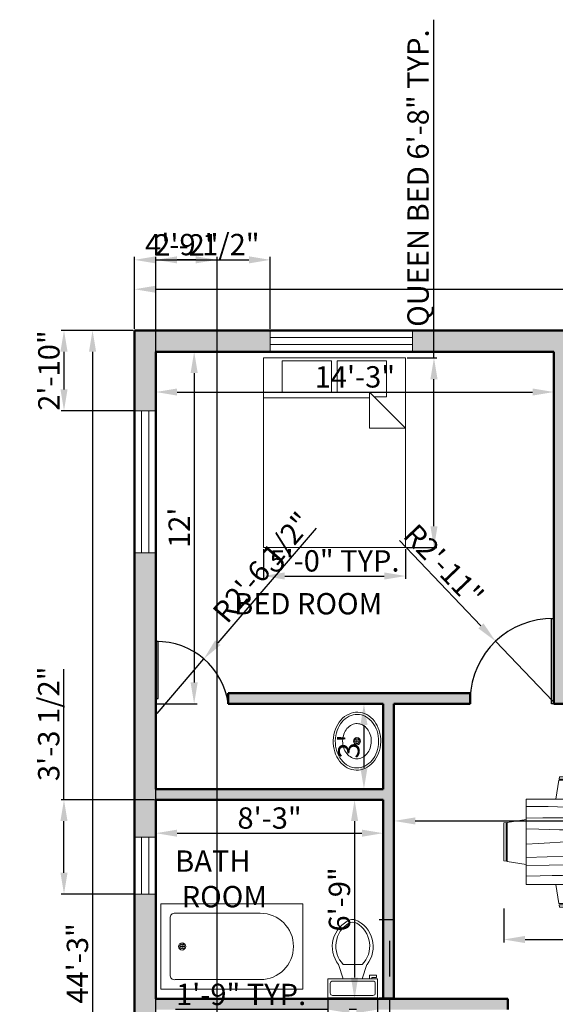
# Model space of a CAD drawing. Units: inches. Extents: x 875413 to 876020, y 447446 to 448210.
# Tile 5 of 8: x 875413 to 875639, y 447795 to 448210. Entities that reach past the tile are written whole.
import ezdxf

# ---------------------------------------------------------------- set-up
doc = ezdxf.new("R2010")
doc.units = ezdxf.units.IN
for name, color, linetype, lineweight in [('A-ANNO-DIMS', 2, 'Continuous', 13), ('A-AREA-IDEN', 7, 'Continuous', 25), ('A-DOOR', 3, 'Continuous', 25), ('A-FLOR-FIXT', 9, 'Continuous', 18), ('A-FURN', 8, 'Continuous', 18), ('A-GLAZ', 4, 'Continuous', 20), ('A-WALL', 7, 'Continuous', 50)]:
    doc.layers.add(name, color=color, linetype=linetype, lineweight=lineweight)
doc.layers.add('A-WALL-PATT', color=18, linetype='Continuous', lineweight=13, true_color=0x000000)
doc.styles.get("Standard").update_dxf_attribs({"font": 'arial.ttf'})
doc.dimstyles.new('ISO-25', dxfattribs={"dimtxt": 9, "dimasz": 9, "dimexe": 1.25, "dimexo": 0.625, "dimtad": 1, "dimdec": 1, "dimrnd": 9, "dimlunit": 3, "dimtxsty": 'Standard', "dimcen": 2.5, "dimadec": 0, "dimazin": 0, "dimtfac": 1, "dimtdec": 1, "dimtmove": 0, "dimatfit": 3, "dimfxl": 1, "dimarcsym": 0})

# ---------------------------------------------------------------- blocks, each defined once
blk = doc.blocks.new('*D1')
at = {"layer": 'A-ANNO-DIMS', "color": 0, "lineweight": -2, "transparency": 16777216}
for p, q in [((875470.7, 448069.39), (875470.7, 448051.77)), ((875638.7, 448069.39), (875638.7, 448051.77)), ((875479.7, 448053.02), (875629.7, 448053.02))]:
    blk.add_line(p, q, dxfattribs=at)
at = {"layer": 'A-ANNO-DIMS', "color": 0, "transparency": 16777216}
for points in [[(875479.7, 448054.52), (875479.7, 448051.52), (875470.7, 448053.02)], [(875629.7, 448054.52), (875629.7, 448051.52), (875638.7, 448053.02)]]:
    blk.add_solid(points, dxfattribs=at)
at = {"layer": 'Defpoints', "color": 0, "transparency": 16777216}
for p in [(875470.7, 448070.02), (875638.7, 448070.02), (875638.7, 448053.02)]:
    blk.add_point(p, dxfattribs=at)
at = {"layer": 'A-ANNO-DIMS', "color": 0, "transparency": 16777216, "insert": (875554.7, 448058.25), "char_height": 9, "attachment_point": 5}
blk.add_mtext('14\'-3"', dxfattribs=at)
blk = doc.blocks.new('*D2')
at = {"layer": 'A-ANNO-DIMS', "color": 0, "lineweight": -2, "transparency": 16777216}
for p, q in [((875471.33, 448070.02), (875488.13, 448070.02)), ((875486.88, 448061.02), (875486.88, 447930.52)), ((875471.33, 447921.52), (875488.13, 447921.52))]:
    blk.add_line(p, q, dxfattribs=at)
at = {"layer": 'A-ANNO-DIMS', "color": 0, "transparency": 16777216}
for points in [[(875485.38, 448061.02), (875488.38, 448061.02), (875486.88, 448070.02)], [(875485.38, 447930.52), (875488.38, 447930.52), (875486.88, 447921.52)]]:
    blk.add_solid(points, dxfattribs=at)
at = {"layer": 'Defpoints', "color": 0, "transparency": 16777216}
for p in [(875470.7, 448070.02), (875470.7, 447921.52), (875486.88, 447921.52)]:
    blk.add_point(p, dxfattribs=at)
at = {"layer": 'A-ANNO-DIMS', "color": 0, "transparency": 16777216, "insert": (875481.73, 447995.77), "char_height": 9, "attachment_point": 5, "rotation": 90}
blk.add_mtext("12'", dxfattribs=at)
blk = doc.blocks.new('*D7')
at = {"layer": 'A-ANNO-DIMS', "color": 0, "lineweight": -2, "transparency": 16777216}
for p, q in [((875566.08, 447921.52), (875557.28, 447921.52)), ((875558.53, 447912.52), (875558.53, 447894.52)), ((875566.08, 447885.52), (875557.28, 447885.52))]:
    blk.add_line(p, q, dxfattribs=at)
at = {"layer": 'A-ANNO-DIMS', "color": 0, "transparency": 16777216}
for points in [[(875557.03, 447912.52), (875560.03, 447912.52), (875558.53, 447921.52)], [(875557.03, 447894.52), (875560.03, 447894.52), (875558.53, 447885.52)]]:
    blk.add_solid(points, dxfattribs=at)
at = {"layer": 'Defpoints', "color": 0, "transparency": 16777216}
for p in [(875566.7, 447921.52), (875558.53, 447885.52), (875566.7, 447885.52)]:
    blk.add_point(p, dxfattribs=at)
at = {"layer": 'A-ANNO-DIMS', "color": 0, "transparency": 16777216, "insert": (875553.31, 447903.52), "char_height": 9, "attachment_point": 5, "rotation": 90}
blk.add_mtext("3'", dxfattribs=at)
blk = doc.blocks.new('*D8')
at = {"layer": 'A-ANNO-DIMS', "color": 0, "lineweight": -2, "transparency": 16777216}
for p, q in [((875566.08, 447881.02), (875553.32, 447881.02)), ((875554.57, 447872.02), (875554.57, 447806.02)), ((875566.08, 447797.02), (875553.32, 447797.02))]:
    blk.add_line(p, q, dxfattribs=at)
at = {"layer": 'A-ANNO-DIMS', "color": 0, "transparency": 16777216}
for points in [[(875553.07, 447872.02), (875556.07, 447872.02), (875554.57, 447881.02)], [(875553.07, 447806.02), (875556.07, 447806.02), (875554.57, 447797.02)]]:
    blk.add_solid(points, dxfattribs=at)
at = {"layer": 'Defpoints', "color": 0, "transparency": 16777216}
for p in [(875566.7, 447881.02), (875554.57, 447797.02), (875566.7, 447797.02)]:
    blk.add_point(p, dxfattribs=at)
at = {"layer": 'A-ANNO-DIMS', "color": 0, "transparency": 16777216, "insert": (875549.35, 447839.02), "char_height": 9, "attachment_point": 5, "rotation": 90}
blk.add_mtext('6\'-9"', dxfattribs=at)
blk = doc.blocks.new('*D9')
at = {"layer": 'A-ANNO-DIMS', "color": 0, "lineweight": -2, "transparency": 16777216}
for p, q in [((875470.7, 447880.39), (875470.7, 447865.69)), ((875566.7, 447880.39), (875566.7, 447865.69)), ((875479.7, 447866.94), (875557.7, 447866.94))]:
    blk.add_line(p, q, dxfattribs=at)
at = {"layer": 'A-ANNO-DIMS', "color": 0, "transparency": 16777216}
for points in [[(875479.7, 447868.44), (875479.7, 447865.44), (875470.7, 447866.94)], [(875557.7, 447868.44), (875557.7, 447865.44), (875566.7, 447866.94)]]:
    blk.add_solid(points, dxfattribs=at)
at = {"layer": 'Defpoints', "color": 0, "transparency": 16777216}
for p in [(875470.7, 447881.02), (875566.7, 447881.02), (875566.7, 447866.94)]:
    blk.add_point(p, dxfattribs=at)
at = {"layer": 'A-ANNO-DIMS', "color": 0, "transparency": 16777216, "insert": (875518.7, 447872.16), "char_height": 9, "attachment_point": 5}
blk.add_mtext('8\'-3"', dxfattribs=at)
blk = doc.blocks.new('*D13')
at = {"layer": 'A-ANNO-DIMS', "color": 0, "lineweight": -2, "transparency": 16777216}
for p, q in [((875571.2, 447920.89), (875571.2, 447870.86)), ((875838.2, 447920.89), (875838.2, 447870.86)), ((875580.2, 447872.11), (875829.2, 447872.11))]:
    blk.add_line(p, q, dxfattribs=at)
at = {"layer": 'A-ANNO-DIMS', "color": 0, "transparency": 16777216}
for points in [[(875580.2, 447873.61), (875580.2, 447870.61), (875571.2, 447872.11)], [(875829.2, 447873.61), (875829.2, 447870.61), (875838.2, 447872.11)]]:
    blk.add_solid(points, dxfattribs=at)
at = {"layer": 'Defpoints', "color": 0, "transparency": 16777216}
for p in [(875571.2, 447921.52), (875838.2, 447921.52), (875838.2, 447872.11)]:
    blk.add_point(p, dxfattribs=at)
at = {"layer": 'A-ANNO-DIMS', "color": 0, "transparency": 16777216, "insert": (875704.7, 447877.33), "char_height": 9, "attachment_point": 5}
blk.add_mtext('22\'-6"', dxfattribs=at)
blk = doc.blocks.new('Bed - Queen')
for p, q in [((0, -80.00003), (0, 0)), ((0, 0), (59.99999, 0)), ((59.99999, 0), (59.99999, -80.00003)), ((7.99999, -1.2), (28.79998, -1.2)), ((7.99999, -14.4), (7.99999, -1.2)), ((28.79998, -1.2), (28.79998, -14.4)), ((31.19999, -1.2), (51.99999, -1.2)), ((31.19999, -14.4), (31.19999, -1.2)), ((51.99999, -1.2), (51.99999, -16.4)), ((0, -14.4), (44.8, -14.4)), ((59.99999, -29.6), (44.8, -14.4)), ((44.8, -14.4), (44.8, -29.6)), ((51.99999, -16.4), (46.79936, -16.4)), ((44.8, -16.8), (0, -16.8)), ((44.8, -29.6), (59.99999, -29.6)), ((59.99999, -80.00003), (0, -80.00003))]:
    blk.add_line(p, q)
blk = doc.blocks.new('Dining Set - 36 x 72 in.')
for p, q in [((-22.2343, 26.00059), (-23.4847, 17.99762)), ((-22.2304, 26), (-5.7608, 26)), ((-22, 27.5), (-22.1562, 26.50042)), ((-5.8416, 26.5), (-22.1534, 26.5)), ((-22, 27.5), (-6, 27.5)), ((-5.8437, 26.49966), (-6, 27.5)), ((-4.5152, 17.99762), (-5.7655, 25.99926)), ((5.7657, 26.00059), (4.5153, 17.99762)), ((5.7696, 26), (22.2392, 26)), ((6, 27.5), (5.8438, 26.50042)), ((22.1584, 26.5), (5.8466, 26.5)), ((6, 27.5), (22, 27.5)), ((22.1563, 26.49966), (22, 27.5)), ((23.4848, 17.99762), (22.2345, 25.99926)), ((36, 18), (-36, 18)), ((-36, 18), (-36, -18)), ((36, -18), (36, 18)), ((-44.0006, 8.23428), (-35.9976, 9.48474)), ((44.0006, 8.23428), (35.9976, 9.48474)), ((-45.5, 8), (-44.5004, 8.15617)), ((-45.5, 8), (-45.5, -8)), ((-44.5, -8.15843), (-44.5, 8.15338)), ((-44, 8.23041), (-44, -8.23915)), ((44, 8.23041), (44, -8.23915)), ((44.5, -8.15843), (44.5, 8.15338)), ((45.5, 8), (44.5005, 8.15617)), ((45.5, 8), (45.5, -8)), ((-44.4997, -8.15631), (-45.5, -8)), ((-35.9976, -9.48476), (-43.9993, -8.2345)), ((35.9976, -9.48476), (43.9993, -8.2345)), ((44.4997, -8.15631), (45.5, -8)), ((-36, -18), (36, -18)), ((-22.2343, -26.0006), (-23.4847, -17.99762)), ((-4.5152, -17.99762), (-5.7655, -25.99928)), ((5.7657, -26.0006), (4.5153, -17.99762)), ((23.4848, -17.99762), (22.2345, -25.99928)), ((-22.2304, -26), (-5.7608, -26)), ((-22, -27.5), (-22.1562, -26.50044)), ((-5.8416, -26.5), (-22.1534, -26.5)), ((-22, -27.5), (-6, -27.5)), ((-5.8437, -26.49967), (-6, -27.5)), ((5.7696, -26), (22.2392, -26)), ((6, -27.5), (5.8438, -26.50044)), ((22.1584, -26.5), (5.8466, -26.5)), ((6, -27.5), (22, -27.5)), ((22.1563, -26.49967), (22, -27.5))]:
    blk.add_line(p, q)
for points in [[(-36, 15), (-31.1772, 14.97754), (-26.8079, 14.91406), (-22.8538, 14.81543), (-19.276, 14.6875), (-16.0362, 14.53613), (-13.0957, 14.36718), (-10.4159, 14.18652), (-7.9583, 14), (-5.6904, 13.81315), (-3.6035, 13.63021), (-1.6954, 13.45508), (0.0365, 13.29166), (1.5945, 13.14388), (2.9811, 13.01562), (4.1988, 12.9108), (5.25, 12.83333), (6.1393, 12.78613), (6.8802, 12.76823), (7.4883, 12.77767), (7.9792, 12.8125), (8.3685, 12.87077), (8.6719, 12.95052), (8.9049, 13.0498), (9.0833, 13.16666), (9.2205, 13.29899), (9.3216, 13.44401), (9.3895, 13.59879), (9.4271, 13.76041), (9.4373, 13.92594), (9.4232, 14.09245), (9.3875, 14.257), (9.3333, 14.41666), (9.2638, 14.56917), (9.1836, 14.71484), (9.0975, 14.85465), (9.0104, 14.98958), (8.9272, 15.1206), (8.8529, 15.2487), (8.7922, 15.37483), (8.75, 15.5), (8.7305, 15.62467), (8.7344, 15.74739), (8.7617, 15.86621), (8.8125, 15.97916), (8.8867, 16.08431), (8.9844, 16.17968), (9.1055, 16.26334), (9.25, 16.33333), (9.4189, 16.38802), (9.6172, 16.42708), (9.8506, 16.45052), (10.125, 16.45833), (10.4463, 16.45052), (10.8203, 16.42708), (11.2529, 16.38802), (11.75, 16.33333), (12.3184, 16.26318), (12.9694, 16.17838), (13.7151, 16.07991), (14.5677, 15.96875), (15.5395, 15.84586), (16.6426, 15.71224), (17.8893, 15.56884), (19.2917, 15.41666), (20.859, 15.25667), (22.5879, 15.08984), (24.4721, 14.91715), (26.5052, 14.73958), (28.6809, 14.5581), (30.9929, 14.3737), (33.4347, 14.18733), (36, 14)], [(-36, 10), (-28.9766, 10.14274), (-23.1725, 10.20442), (-18.4241, 10.19775), (-14.5677, 10.13541), (-11.4399, 10.03011), (-8.877, 9.89453), (-6.7154, 9.74137), (-4.7917, 9.58333), (-2.9698, 9.43082), (-1.2246, 9.28515), (0.4415, 9.14534), (2.026, 9.01041), (3.5266, 8.87939), (4.9408, 8.7513), (6.266, 8.62516), (7.5, 8.5), (8.6411, 8.37549), (9.6914, 8.2539), (10.6538, 8.13818), (11.5312, 8.03125), (12.3267, 7.93603), (13.043, 7.85547), (13.6831, 7.79248), (14.25, 7.75), (14.7471, 7.7303), (15.1797, 7.73307), (15.5537, 7.75732), (15.875, 7.80208), (16.1494, 7.86637), (16.3828, 7.94922), (16.5811, 8.04964), (16.75, 8.16666), (16.8944, 8.29915), (17.0143, 8.44531), (17.1089, 8.60319), (17.1771, 8.77083), (17.218, 8.94629), (17.2305, 9.1276), (17.2137, 9.31282), (17.1667, 9.5), (17.0895, 9.6875), (16.987, 9.875), (16.8649, 10.0625), (16.7292, 10.25), (16.5856, 10.4375), (16.4401, 10.625), (16.2985, 10.8125), (16.1667, 11), (16.05, 11.18733), (15.9518, 11.3737), (15.8752, 11.5581), (15.8229, 11.73958), (15.798, 11.91715), (15.8034, 12.08984), (15.842, 12.25667), (15.9167, 12.41666), (16.0295, 12.56836), (16.1784, 12.70833), (16.3605, 12.83268), (16.5729, 12.9375), (16.8127, 13.01888), (17.0768, 13.07291), (17.3625, 13.0957), (17.6667, 13.08333), (17.9894, 13.03312), (18.3418, 12.94726), (18.7382, 12.82918), (19.1927, 12.68229), (19.7195, 12.51001), (20.3327, 12.31575), (21.0465, 12.10294), (21.875, 11.875), (22.8357, 11.63354), (23.959, 11.37304), (25.2786, 11.08618), (26.8282, 10.76562), (28.6414, 10.40405), (30.752, 9.99414), (33.1936, 9.52856), (36, 9)], [(-36, 5.5), (-30.7157, 5.3348), (-26.069, 5.20963), (-21.9946, 5.11767), (-18.4271, 5.05208), (-15.3009, 5.00602), (-12.5508, 4.97265), (-10.1112, 4.94515), (-7.9167, 4.91666), (-5.909, 4.88167), (-4.0586, 4.83984), (-2.3429, 4.79215), (-0.7396, 4.73958), (0.7739, 4.6831), (2.22, 4.6237), (3.6213, 4.56233), (5, 4.5), (6.373, 4.43782), (7.7344, 4.3776), (9.0723, 4.32129), (10.375, 4.27083), (11.6309, 4.22819), (12.8281, 4.19531), (13.9551, 4.17415), (15, 4.16666), (15.954, 4.17448), (16.819, 4.19791), (17.6001, 4.23698), (18.3021, 4.29166), (18.9299, 4.36198), (19.4883, 4.44791), (19.9823, 4.54948), (20.4167, 4.66666), (20.7969, 4.79899), (21.1302, 4.94401), (21.4245, 5.09879), (21.6875, 5.26041), (21.9271, 5.42594), (22.1511, 5.59245), (22.3672, 5.757), (22.5834, 5.91666), (22.8065, 6.06868), (23.0404, 6.21093), (23.2879, 6.34147), (23.5521, 6.45833), (23.8358, 6.55957), (24.142, 6.64323), (24.4735, 6.70735), (24.8334, 6.75), (25.2235, 6.76969), (25.642, 6.76692), (26.0858, 6.74267), (26.5521, 6.69791), (27.0379, 6.63362), (27.5404, 6.55078), (28.0565, 6.45036), (28.5834, 6.33333), (29.1242, 6.19987), (29.7071, 6.04687), (30.3661, 5.87044), (31.1354, 5.66666), (32.0493, 5.43164), (33.142, 5.16146), (34.4475, 4.85221), (36, 4.5)], [(-36, -1), (-30.7915, -0.6591), (-26.0195, -0.38216), (-21.6519, -0.16284), (-17.6563, 0.00521), (-14.0005, 0.12833), (-10.6523, 0.21289), (-7.5796, 0.26522), (-4.75, 0.29166), (-2.134, 0.29793), (0.2878, 0.28711), (2.5317, 0.26163), (4.6146, 0.22396), (6.5529, 0.17651), (8.3633, 0.12174), (10.0623, 0.06209), (11.6667, 0), (13.1899, -0.06201), (14.6341, -0.1211), (15.9982, -0.17432), (17.2813, -0.21875), (18.4823, -0.25147), (19.6003, -0.26953), (20.6343, -0.27002), (21.5834, -0.25), (22.4481, -0.20768), (23.2357, -0.14584), (23.9549, -0.06836), (24.6146, 0.02083), (25.2235, 0.11784), (25.7904, 0.21875), (26.3241, 0.31966), (26.8334, 0.41666), (27.3265, 0.50618), (27.8099, 0.58593), (28.2894, 0.65397), (28.7709, 0.70833), (29.2601, 0.74707), (29.763, 0.76823), (30.2855, 0.76985), (30.8334, 0.75), (31.4088, 0.70784), (31.9994, 0.64713), (32.589, 0.57275), (33.1615, 0.48958), (33.7008, 0.4025), (34.1908, 0.3164), (34.6153, 0.23616), (34.9584, 0.16666), (35.2099, 0.11165), (35.3848, 0.07031), (35.504, 0.04069), (35.5886, 0.02083), (35.6594, 0.00879), (35.7377, 0.0026), (35.8442, 0.00032), (36, 0)], [(-36, -6.5), (-27.1843, -6.31267), (-20.084, -6.1263), (-14.469, -5.9419), (-10.1094, -5.76042), (-6.7752, -5.58285), (-4.2363, -5.41016), (-2.2629, -5.24333), (-0.625, -5.08334), (0.8708, -4.93099), (2.2715, -4.78646), (3.5872, -4.64974), (4.8281, -4.52084), (6.0046, -4.39974), (7.127, -4.28646), (8.2053, -4.18099), (9.25, -4.08334), (10.2705, -3.99382), (11.2734, -3.91407), (12.2647, -3.84603), (13.25, -3.79167), (14.2354, -3.75293), (15.2266, -3.73177), (16.2295, -3.73015), (17.25, -3.75), (18.2912, -3.79248), (19.3451, -3.85547), (20.4009, -3.93604), (21.4479, -4.03125), (22.4754, -4.13819), (23.4727, -4.25391), (24.4289, -4.37549), (25.3334, -4.5), (26.1785, -4.62492), (26.9694, -4.74935), (27.7145, -4.87281), (28.4219, -4.99479), (29.1, -5.11483), (29.7572, -5.23242), (30.4016, -5.34709), (31.0417, -5.45834), (31.6837, -5.56437), (32.3262, -5.65821), (32.9658, -5.73153), (33.599, -5.77604), (34.2224, -5.78345), (34.8327, -5.74545), (35.4264, -5.65373), (36, -5.5)], [(-36, -10), (-26.4022, -9.81299), (-18.4675, -9.62891), (-11.9839, -9.45069), (-6.7396, -9.28125), (-2.5226, -9.12354), (0.8789, -8.98047), (3.6769, -8.85498), (6.0833, -8.75), (8.2767, -8.66765), (10.3021, -8.60677), (12.1712, -8.56543), (13.8958, -8.54167), (15.4876, -8.53353), (16.9583, -8.53907), (18.3197, -8.55632), (19.5834, -8.58334), (20.7616, -8.61841), (21.8685, -8.66081), (22.9188, -8.71004), (23.9271, -8.76563), (24.9081, -8.82707), (25.8763, -8.89388), (26.8465, -8.96558), (27.8334, -9.04167), (28.8474, -9.12118), (29.8828, -9.20117), (30.93, -9.27824), (31.9792, -9.34896), (33.0205, -9.40991), (34.0443, -9.45768), (35.0407, -9.48885), (36, -9.5)], [(-36, -14.5), (-30.0881, -14.33513), (-25.0332, -14.21224), (-20.7312, -14.12647), (-17.0781, -14.07292), (-13.97, -14.04671), (-11.3027, -14.04297), (-8.9724, -14.05681), (-6.875, -14.08334), (-4.9224, -14.11833), (-3.0905, -14.16016), (-1.3709, -14.20785), (0.2448, -14.26042), (1.7647, -14.3169), (3.1973, -14.3763), (4.5507, -14.43767), (5.8333, -14.5), (7.0554, -14.5621), (8.235, -14.62175), (9.3922, -14.67652), (10.5469, -14.72396), (11.7192, -14.76164), (12.929, -14.78711), (14.1965, -14.79794), (15.5417, -14.79167), (16.9933, -14.76424), (18.6152, -14.70508), (20.4804, -14.60197), (22.6615, -14.44271), (25.2312, -14.21509), (28.2624, -13.9069), (31.8277, -13.50594), (36, -13)]]:
    blk.add_lwpolyline(points)
blk = doc.blocks.new('Sink - Oval top')
for p, q in [((-1, 0), (1, 0)), ((0, 1), (0, -1))]:
    blk.add_line(p, q)
for points in [[(-12.23, 0.39, 0.117634), (-11.46, -3.36, 0.104469), (-8.88, -6.8, 0.090016), (-5.08, -9.07, 0.08192), (-0.32, -10.02, 0.08192), (4.49, -9.38, 0.090016), (8.42, -7.36, 0.104469), (11.22, -4.09, 0.117634), (12.23, -0.39, 0.117634), (11.46, 3.36, 0.104469), (8.88, 6.8, 0.090016), (5.08, 9.07, 0.08192), (0.32, 10.02, 0.08192), (-4.49, 9.38, 0.090016), (-8.42, 7.36, 0.104469), (-11.22, 4.09, 0.117634)], [(-11.29, 0.16, 0.118622), (-10.52, -3.25, 0.104678), (-8.07, -6.36, 0.089562), (-4.54, -8.37, 0.081185), (-0.13, -9.15, 0.081185), (4.3, -8.49, 0.089562), (7.89, -6.58, 0.104678), (10.42, -3.55, 0.118622), (11.29, -0.16, 0.118622), (10.52, 3.25, 0.104678), (8.07, 6.36, 0.089562), (4.54, 8.37, 0.081185), (0.13, 9.15, 0.081185), (-4.3, 8.49, 0.089562), (-7.89, 6.58, 0.104678), (-10.42, 3.55, 0.118622)], [(-7.42, 0.08, 0.118283), (-6.91, -2.17, 0.104607), (-5.29, -4.21, 0.089718), (-2.97, -5.53, 0.081436), (-0.07, -6.04, 0.081436), (2.84, -5.59, 0.089718), (5.2, -4.33, 0.104607), (6.86, -2.32, 0.118283), (7.42, -0.08, 0.118283), (6.91, 2.17, 0.104607), (5.29, 4.21, 0.089718), (2.97, 5.53, 0.081436), (0.07, 6.04, 0.081436), (-2.84, 5.59, 0.089718), (-5.2, 4.33, 0.104607), (-6.86, 2.32, 0.118283)]]:
    blk.add_lwpolyline(points, format="xyb", close=True)
for radius in [1.5, 1]:
    blk.add_circle((0, 0), radius)
blk = doc.blocks.new('Toilet - top')
for p, q in [((9.5, -6), (9.5, -2)), ((-8, -8.5), (-8, -8)), ((-7, -8), (-7, -9.5)), ((-4, -8), (-6, -14)), ((4, -8), (6, -14)), ((-10, -8.5), (-8, -8.5)), ((-10, -9.5), (-10, -8.5)), ((-7, -9.5), (-10, -9.5)), ((4, -14), (-4, -14))]:
    blk.add_line(p, q)
blk.add_lwpolyline([(10.5, -8), (10.5, 0), (-10.5, 0), (-10.5, -8)], close=True)
for points in [[(-9.5, -2), (-9.5, -6)], [(8.5, -1), (-8.5, -1)], [(-8.5, -7), (8.5, -7)]]:
    blk.add_lwpolyline(points)
for centre, radius, start, end in [((-8.62, -1.88), 0.884, 81.8699, 188.1301), ((8.62, -1.88), 0.884, 351.8699, 98.1301), ((-8.62, -6.12), 0.884, 171.8699, 278.1301), ((8.62, -6.12), 0.884, 261.8699, 8.1301), ((3.52, -21.58), 12.17, 141.4691, 247.9714), ((4.2, -21.82), 11.33, 136.3677, 238.9468), ((-3.52, -21.58), 12.17, 292.0284, 38.5307), ((-4.2, -21.82), 11.33, 301.053, 43.6321), ((0, -27.88), 4, 245.7318, 294.2682), ((0, -29), 4, 254.8605, 285.1395)]:
    blk.add_arc(centre, radius, start, end)
blk = doc.blocks.new('Bath Tub - 26 x 60 in.')
for p, q in [((8, -18), (10, -18)), ((9, -17), (9, -19))]:
    blk.add_line(p, q)
blk.add_lwpolyline([(0, -36), (0, 0), (60, 0), (60, -36)], close=True)
for points in [[(6, -4), (42, -4)], [(4, -30), (4, -6)], [(42, -32), (6, -32)]]:
    blk.add_lwpolyline(points)
for radius in [1.5, 1]:
    blk.add_circle((9, -18), radius)
for centre, radius, start, end in [((5.75, -5.75), 1.77, 81.8699, 188.1301), ((42, -18), 14, 270, 90), ((5.75, -30.25), 1.77, 171.8699, 278.1301)]:
    blk.add_arc(centre, radius, start, end)
blk = doc.blocks.new('*D37')
at = {"layer": 'A-ANNO-DIMS', "color": 0, "lineweight": -2, "transparency": 16777216}
for p, q in [((875461.7, 448079.64), (875461.7, 448097.63)), ((875470.7, 448096.38), (875926.7, 448096.38)), ((875935.7, 448079.64), (875935.7, 448097.63))]:
    blk.add_line(p, q, dxfattribs=at)
at = {"layer": 'A-ANNO-DIMS', "color": 0, "transparency": 16777216}
for points in [[(875470.7, 448097.88), (875470.7, 448094.88), (875461.7, 448096.38)], [(875926.7, 448097.88), (875926.7, 448094.88), (875935.7, 448096.38)]]:
    blk.add_solid(points, dxfattribs=at)
at = {"layer": 'Defpoints', "color": 0, "transparency": 16777216}
for p in [(875935.7, 448096.38), (875461.7, 448079.02), (875935.7, 448079.02)]:
    blk.add_point(p, dxfattribs=at)
at = {"layer": 'A-ANNO-DIMS', "color": 0, "transparency": 16777216, "insert": (875698.7, 448101.6), "char_height": 9, "attachment_point": 5}
blk.add_mtext('39\'-9"', dxfattribs=at)
blk = doc.blocks.new('*D38')
at = {"layer": 'A-ANNO-DIMS', "color": 0, "lineweight": -2, "transparency": 16777216}
for p, q in [((875461.08, 448079.02), (875442.76, 448079.02)), ((875444.01, 448070.02), (875444.01, 447554.02)), ((875461.08, 447545.02), (875442.76, 447545.02))]:
    blk.add_line(p, q, dxfattribs=at)
at = {"layer": 'A-ANNO-DIMS', "color": 0, "transparency": 16777216}
for points in [[(875442.51, 448070.02), (875445.51, 448070.02), (875444.01, 448079.02)], [(875442.51, 447554.02), (875445.51, 447554.02), (875444.01, 447545.02)]]:
    blk.add_solid(points, dxfattribs=at)
at = {"layer": 'Defpoints', "color": 0, "transparency": 16777216}
for p in [(875461.7, 448079.02), (875444.01, 447545.02), (875461.7, 447545.02)]:
    blk.add_point(p, dxfattribs=at)
at = {"layer": 'A-ANNO-DIMS', "color": 0, "transparency": 16777216, "insert": (875438.78, 447812.02), "char_height": 9, "attachment_point": 5, "rotation": 90}
blk.add_mtext('44\'-3"', dxfattribs=at)
blk = doc.blocks.new('WIN-60IN')
for p, q in [((0, 9), (0, 0)), ((60, 9), (60, 0)), ((60, 6), (0, 6)), ((60, 3), (0, 3))]:
    blk.add_line(p, q)
blk = doc.blocks.new('WIN-24IN')
for p, q in [((0, 24), (9, 24)), ((3, 0), (3, 24)), ((6, 0), (6, 24)), ((0, 0), (9, 0))]:
    blk.add_line(p, q)
blk = doc.blocks.new('*D45')
at = {"layer": 'A-ANNO-DIMS', "color": 0, "lineweight": -2, "transparency": 16777216}
for p, q in [((875588.08, 448067.42), (875588.08, 448210.07)), ((875576.71, 448067.42), (875589.33, 448067.42)), ((875588.08, 447996.42), (875588.08, 448058.42)), ((875576.71, 447987.42), (875589.33, 447987.42))]:
    blk.add_line(p, q, dxfattribs=at)
at = {"layer": 'A-ANNO-DIMS', "color": 0, "transparency": 16777216}
for points in [[(875586.58, 448058.42), (875589.58, 448058.42), (875588.08, 448067.42)], [(875586.58, 447996.42), (875589.58, 447996.42), (875588.08, 447987.42)]]:
    blk.add_solid(points, dxfattribs=at)
at = {"layer": 'Defpoints', "color": 0, "transparency": 16777216}
for p in [(875576.08, 448067.42), (875588.08, 448067.42), (875576.08, 447987.42)]:
    blk.add_point(p, dxfattribs=at)
at = {"layer": 'A-ANNO-DIMS', "color": 0, "transparency": 16777216, "insert": (875582.53, 448143.25), "char_height": 9, "attachment_point": 5, "rotation": 90}
blk.add_mtext('QUEEN BED 6\'-8" TYP.', dxfattribs=at)
blk = doc.blocks.new('*D46')
at = {"layer": 'A-ANNO-DIMS', "color": 0, "lineweight": -2, "transparency": 16777216}
for p, q in [((875516.08, 447986.8), (875516.08, 447974.17)), ((875576.08, 447986.8), (875576.08, 447974.17)), ((875525.08, 447975.42), (875567.08, 447975.42))]:
    blk.add_line(p, q, dxfattribs=at)
at = {"layer": 'A-ANNO-DIMS', "color": 0, "transparency": 16777216}
for points in [[(875525.08, 447976.92), (875525.08, 447973.92), (875516.08, 447975.42)], [(875567.08, 447976.92), (875567.08, 447973.92), (875576.08, 447975.42)]]:
    blk.add_solid(points, dxfattribs=at)
at = {"layer": 'Defpoints', "color": 0, "transparency": 16777216}
for p in [(875516.08, 447987.42), (875576.08, 447987.42), (875576.08, 447975.42)]:
    blk.add_point(p, dxfattribs=at)
at = {"layer": 'A-ANNO-DIMS', "color": 0, "transparency": 16777216, "insert": (875546.08, 447980.64), "char_height": 9, "attachment_point": 5}
blk.add_mtext('5\'-0" TYP.', dxfattribs=at)
blk = doc.blocks.new('*D49')
at = {"layer": 'A-ANNO-DIMS', "color": 0, "lineweight": -2, "transparency": 16777216}
for p, q in [((875564.95, 447830.56), (875570.53, 447830.56)), ((875569.28, 447821.56), (875569.28, 447806.52)), ((875564.95, 447797.52), (875570.53, 447797.52)), ((875569.28, 447797.52), (875569.28, 447707.6))]:
    blk.add_line(p, q, dxfattribs=at)
at = {"layer": 'A-ANNO-DIMS', "color": 0, "transparency": 16777216}
for points in [[(875567.78, 447821.56), (875570.78, 447821.56), (875569.28, 447830.56)], [(875567.78, 447806.52), (875570.78, 447806.52), (875569.28, 447797.52)]]:
    blk.add_solid(points, dxfattribs=at)
at = {"layer": 'Defpoints', "color": 0, "transparency": 16777216}
for p in [(875564.32, 447830.56), (875564.32, 447797.52), (875569.28, 447797.52)]:
    blk.add_point(p, dxfattribs=at)
at = {"layer": 'A-ANNO-DIMS', "color": 0, "transparency": 16777216, "insert": (875564, 447748.06), "char_height": 9, "attachment_point": 5, "rotation": 90}
blk.add_mtext('WC 2\'-9" TYP.', dxfattribs=at)
blk = doc.blocks.new('*D50')
at = {"layer": 'A-ANNO-DIMS', "color": 0, "lineweight": -2, "transparency": 16777216}
for p, q in [((875543.32, 447796.89), (875543.32, 447791.31)), ((875564.32, 447796.89), (875564.32, 447791.31)), ((875543.32, 447792.56), (875479.06, 447792.56)), ((875555.32, 447792.56), (875552.32, 447792.56))]:
    blk.add_line(p, q, dxfattribs=at)
at = {"layer": 'A-ANNO-DIMS', "color": 0, "transparency": 16777216}
for points in [[(875552.32, 447794.06), (875552.32, 447791.06), (875543.32, 447792.56)], [(875555.32, 447794.06), (875555.32, 447791.06), (875564.32, 447792.56)]]:
    blk.add_solid(points, dxfattribs=at)
at = {"layer": 'Defpoints', "color": 0, "transparency": 16777216}
for p in [(875543.32, 447797.52), (875564.32, 447797.52), (875543.32, 447792.56)]:
    blk.add_point(p, dxfattribs=at)
at = {"layer": 'A-ANNO-DIMS', "color": 0, "transparency": 16777216, "insert": (875506.69, 447797.78), "char_height": 9, "attachment_point": 5}
blk.add_mtext('1\'-9" TYP.', dxfattribs=at)
blk = doc.blocks.new('*D53')
at = {"layer": 'A-ANNO-DIMS', "color": 0, "lineweight": -2, "transparency": 16777216}
for p, q in [((875617.53, 447835.12), (875617.53, 447820.85)), ((875708.53, 447835.12), (875708.53, 447820.85)), ((875626.53, 447822.1), (875699.53, 447822.1)), ((875708.53, 447822.1), (875817.7, 447822.1))]:
    blk.add_line(p, q, dxfattribs=at)
at = {"layer": 'A-ANNO-DIMS', "color": 0, "transparency": 16777216}
for points in [[(875626.53, 447823.6), (875626.53, 447820.6), (875617.53, 447822.1)], [(875699.53, 447823.6), (875699.53, 447820.6), (875708.53, 447822.1)]]:
    blk.add_solid(points, dxfattribs=at)
at = {"layer": 'Defpoints', "color": 0, "transparency": 16777216}
for p in [(875617.53, 447835.75), (875708.53, 447835.75), (875708.53, 447822.1)]:
    blk.add_point(p, dxfattribs=at)
at = {"layer": 'A-ANNO-DIMS', "color": 0, "transparency": 16777216, "insert": (875767.62, 447827.38), "char_height": 9, "attachment_point": 5}
blk.add_mtext('DINING SET 7\'-7"', dxfattribs=at)
blk = doc.blocks.new('*D67')
at = {"layer": 'A-ANNO-DIMS', "color": 0, "lineweight": -2, "transparency": 16777216}
for p, q in [((875461.7, 448079.64), (875461.7, 448110.02)), ((875470.7, 448108.77), (875509.96, 448108.77)), ((875518.96, 448079.64), (875518.96, 448110.02))]:
    blk.add_line(p, q, dxfattribs=at)
at = {"layer": 'A-ANNO-DIMS', "color": 0, "transparency": 16777216}
for points in [[(875470.7, 448110.27), (875470.7, 448107.27), (875461.7, 448108.77)], [(875509.96, 448110.27), (875509.96, 448107.27), (875518.96, 448108.77)]]:
    blk.add_solid(points, dxfattribs=at)
at = {"layer": 'Defpoints', "color": 0, "transparency": 16777216}
for p in [(875518.96, 448108.77), (875461.7, 448079.02), (875518.96, 448079.02)]:
    blk.add_point(p, dxfattribs=at)
at = {"layer": 'A-ANNO-DIMS', "color": 0, "transparency": 16777216, "insert": (875490.33, 448114.05), "char_height": 9, "attachment_point": 5}
blk.add_mtext('4\'-9 1/2"', dxfattribs=at)
blk = doc.blocks.new('*D69')
at = {"layer": 'A-ANNO-DIMS', "color": 0, "lineweight": -2, "transparency": 16777216}
for p, q in [((875461.08, 448079.02), (875430.7, 448079.02)), ((875431.95, 448070.02), (875431.95, 448054.13)), ((875461.08, 448045.13), (875430.7, 448045.13))]:
    blk.add_line(p, q, dxfattribs=at)
at = {"layer": 'A-ANNO-DIMS', "color": 0, "transparency": 16777216}
for points in [[(875430.45, 448070.02), (875433.45, 448070.02), (875431.95, 448079.02)], [(875430.45, 448054.13), (875433.45, 448054.13), (875431.95, 448045.13)]]:
    blk.add_solid(points, dxfattribs=at)
at = {"layer": 'Defpoints', "color": 0, "transparency": 16777216}
for p in [(875461.7, 448079.02), (875431.95, 448045.13), (875461.7, 448045.13)]:
    blk.add_point(p, dxfattribs=at)
at = {"layer": 'A-ANNO-DIMS', "color": 0, "transparency": 16777216, "insert": (875426.73, 448062.08), "char_height": 9, "attachment_point": 5, "rotation": 90}
blk.add_mtext('2\'-10"', dxfattribs=at)
blk = doc.blocks.new('*D71')
at = {"layer": 'A-ANNO-DIMS', "color": 0, "lineweight": -2, "transparency": 16777216}
for p, q in [((875431.95, 447881.02), (875431.95, 447936.16)), ((875470.08, 447881.02), (875430.7, 447881.02)), ((875431.95, 447850.29), (875431.95, 447872.02)), ((875461.08, 447841.29), (875430.7, 447841.29))]:
    blk.add_line(p, q, dxfattribs=at)
at = {"layer": 'A-ANNO-DIMS', "color": 0, "transparency": 16777216}
for points in [[(875430.45, 447872.02), (875433.45, 447872.02), (875431.95, 447881.02)], [(875430.45, 447850.29), (875433.45, 447850.29), (875431.95, 447841.29)]]:
    blk.add_solid(points, dxfattribs=at)
at = {"layer": 'Defpoints', "color": 0, "transparency": 16777216}
for p in [(875431.95, 447881.02), (875470.7, 447881.02), (875461.7, 447841.29)]:
    blk.add_point(p, dxfattribs=at)
at = {"layer": 'A-ANNO-DIMS', "color": 0, "transparency": 16777216, "insert": (875426.67, 447913.09), "char_height": 9, "attachment_point": 5, "rotation": 90}
blk.add_mtext('3\'-3 1/2"', dxfattribs=at)
blk = doc.blocks.new('*D82')
at = {"layer": 'A-ANNO-DIMS', "color": 0, "lineweight": -2, "transparency": 16777216}
for p, q in [((875470.7, 447554.64), (875470.7, 448110.02)), ((875487.52, 448108.77), (875479.7, 448108.77)), ((875496.52, 447585.21), (875496.52, 448110.02))]:
    blk.add_line(p, q, dxfattribs=at)
at = {"layer": 'A-ANNO-DIMS', "color": 0, "transparency": 16777216}
for points in [[(875479.7, 448110.27), (875479.7, 448107.27), (875470.7, 448108.77)], [(875487.52, 448110.27), (875487.52, 448107.27), (875496.52, 448108.77)]]:
    blk.add_solid(points, dxfattribs=at)
at = {"layer": 'Defpoints', "color": 0, "transparency": 16777216}
for p in [(875470.7, 448108.77), (875496.52, 447584.59), (875470.7, 447554.02)]:
    blk.add_point(p, dxfattribs=at)
at = {"layer": 'A-ANNO-DIMS', "color": 0, "transparency": 16777216, "insert": (875483.61, 448113.91), "char_height": 9, "attachment_point": 5}
blk.add_mtext('2\'-2"', dxfattribs=at)
blk = doc.blocks.new('*D95')
at = {"layer": 'A-ANNO-DIMS', "color": 0, "lineweight": -2, "transparency": 16777216}
for p, q in [((875573.55, 447990.43), (875607.89, 447954.39)), ((875638.2, 447922.58), (875614.1, 447947.88))]:
    blk.add_line(p, q, dxfattribs=at)
at = {"layer": 'A-ANNO-DIMS', "color": 0, "transparency": 16777216}
blk.add_solid([(875608.98, 447955.43), (875606.81, 447953.36), (875614.1, 447947.88)], dxfattribs=at)
at = {"layer": 'Defpoints', "color": 0, "transparency": 16777216}
for p in [(875614.1, 447947.88), (875638.2, 447922.58)]:
    blk.add_point(p, dxfattribs=at)
at = {"layer": 'A-ANNO-DIMS', "color": 0, "transparency": 16777216, "insert": (875591.34, 447979.22), "char_height": 9, "attachment_point": 5, "rotation": 313.6195}
blk.add_mtext('R2\'-11"', dxfattribs=at)
blk = doc.blocks.new('*D99')
at = {"layer": 'A-ANNO-DIMS', "color": 0, "lineweight": -2, "transparency": 16777216}
for p, q in [((875538.37, 447995.65), (875496.84, 447947.28)), ((875471.2, 447917.42), (875490.97, 447940.45))]:
    blk.add_line(p, q, dxfattribs=at)
at = {"layer": 'A-ANNO-DIMS', "color": 0, "transparency": 16777216}
blk.add_solid([(875495.7, 447948.25), (875497.97, 447946.3), (875490.97, 447940.45)], dxfattribs=at)
at = {"layer": 'Defpoints', "color": 0, "transparency": 16777216}
for p in [(875490.97, 447940.45), (875471.2, 447917.42)]:
    blk.add_point(p, dxfattribs=at)
at = {"layer": 'A-ANNO-DIMS', "color": 0, "transparency": 16777216, "insert": (875516.53, 447978.32), "char_height": 9, "attachment_point": 5, "rotation": 49.3496}
blk.add_mtext('R2\'-6 1/2"', dxfattribs=at)

msp = doc.modelspace()

# ---------------------------------------------------------------- hatches: boundary and pattern name
at = {"layer": 'A-WALL-PATT'}
h = msp.add_hatch(color=256, dxfattribs=at)
h.dxf.hatch_style = 1
h.paths.add_polyline_path([(875470.7, 447985.13), (875461.7, 447985.13), (875461.7, 447865.29), (875470.7, 447865.29), (875470.7, 447881.02), (875566.7, 447881.02), (875566.7, 447797.02), (875571.2, 447797.02), (875571.2, 447885.52), (875571.2, 447921.52), (875603.29, 447921.52), (875603.29, 447926.02), (875501.27, 447926.02), (875501.27, 447921.52), (875566.7, 447921.52), (875566.7, 447885.52), (875470.7, 447885.52), (875470.7, 447921.52), (875470.7, 447926.02)])
h.paths.add_polyline_path([(875470.7, 448070.02), (875518.96, 448070.02), (875518.96, 448079.02), (875461.7, 448079.02), (875461.7, 448045.13), (875470.7, 448045.13)])
h.paths.add_polyline_path([(875819.9, 448079.02), (875578.96, 448079.02), (875578.96, 448070.02), (875638.7, 448070.02), (875638.7, 447921.52), (875643.2, 447921.52), (875643.2, 448070.02), (875763.2, 448070.02), (875763.2, 447921.52), (875767.7, 447921.52), (875767.7, 448070.02), (875819.9, 448070.02)])
h.paths.add_polyline_path([(875935.7, 447978.92), (875926.7, 447978.92), (875926.7, 447926.02), (875926.7, 447921.52), (875926.7, 447885.52), (875842.7, 447885.52), (875842.7, 447921.52), (875899.7, 447921.52), (875899.7, 447926.02), (875805.34, 447926.02), (875805.34, 447921.52), (875838.2, 447921.52), (875838.2, 447885.52), (875838.2, 447797.02), (875689.7, 447797.02), (875689.7, 447792.52), (875842.7, 447792.52), (875842.7, 447881.02), (875926.7, 447881.02), (875926.7, 447857.16), (875935.7, 447857.16)])
h.paths.add_polyline_path([(875935.7, 448079.02), (875879.9, 448079.02), (875879.9, 448070.02), (875926.7, 448070.02), (875926.7, 448038.92), (875935.7, 448038.92)])
h.paths.add_polyline_path([(875935.7, 447833.16), (875926.7, 447833.16), (875926.7, 447797.02), (875842.7, 447797.02), (875842.7, 447792.52), (875926.7, 447792.52), (875926.7, 447756.52), (875935.7, 447756.52)])
h.paths.add_polyline_path([(875935.7, 447732.52), (875926.7, 447732.52), (875926.7, 447692.75, -0.007222), (875926.81, 447692.41, -0.08192), (875927.45, 447687.6, -0.071798), (875926.7, 447683.4), (875926.7, 447672.52), (875808.63, 447672.52), (875808.63, 447668.02), (875926.7, 447668.02), (875926.7, 447663.19), (875935.7, 447663.19)])
h.paths.add_polyline_path([(875842.7, 447792.52), (875838.2, 447792.52), (875838.2, 447704.02), (875842.7, 447704.02)])
h.paths.add_polyline_path([(875470.7, 447792.52), (875619.2, 447792.52), (875619.2, 447797.02), (875470.7, 447797.02), (875470.7, 447841.29), (875461.7, 447841.29), (875461.7, 447764.71), (875470.7, 447764.71)])
h.paths.add_polyline_path([(875619.2, 447760.51), (875616.95, 447760.51, -0.018388), (875614.7, 447760.37), (875614.7, 447672.52), (875470.7, 447672.52), (875470.7, 447704.71), (875461.7, 447704.71), (875461.7, 447640.7), (875470.7, 447640.7), (875470.7, 447668.02), (875619.2, 447668.02)])
h.paths.add_polyline_path([(875511.12, 447554.02), (875470.7, 447554.02), (875470.7, 447580.7), (875461.7, 447580.7), (875461.7, 447545.02), (875511.12, 447545.02)])
h.paths.add_polyline_path([(875656.47, 447554.02), (875620.05, 447554.02, -0.057036), (875616.67, 447553.74, -0.040891), (875614.26, 447554.02), (875571.12, 447554.02), (875571.12, 447545.02), (875656.47, 447545.02)])
h.paths.add_polyline_path([(875643.2, 447613.27), (875685.21, 447613.27), (875685.21, 447617.77), (875685.21, 447623.8), (875680.71, 447623.8), (875680.71, 447617.77), (875618.23, 447617.77), (875618.23, 447623.8), (875613.73, 447623.8), (875613.73, 447617.77), (875613.73, 447613.27), (875638.7, 447613.27), (875638.7, 447554.02), (875643.2, 447554.02)])
h.paths.add_polyline_path([(875694.2, 447760.28), (875689.7, 447760.28), (875689.7, 447668.02), (875748.63, 447668.02), (875748.63, 447672.52), (875694.2, 447672.52)])

# ---------------------------------------------------------------- linework, layer by layer
at = {"layer": 'A-DOOR'}
for p, q in [((875637.7, 447921.52), (875637.7, 447957.52)), ((875637.7, 447957.52), (875638.7, 447957.52)), ((875471.7, 447947.77), (875470.7, 447947.77)), ((875471.7, 447923.77), (875471.7, 447947.77)), ((875470.7, 447923.77), (875471.7, 447923.77)), ((875638.7, 447921.52), (875637.7, 447921.52))]:
    msp.add_line(p, q, dxfattribs=at)
for centre, radius, start, end in [((875638.2, 447922.58), 34.94, 89.18, 178.059), ((875471.2, 447917.42), 30.35, 7.7553, 90.944)]:
    msp.add_arc(centre, radius, start, end, dxfattribs=at)
at = {"layer": 'A-WALL'}
for p, q in [((875935.7, 448079.02), (875461.7, 448079.02)), ((875461.7, 448079.02), (875461.7, 447545.02)), ((875470.7, 448070.02), (875470.7, 447926.02)), ((875638.7, 448070.02), (875470.7, 448070.02)), ((875638.7, 448070.02), (875638.7, 447921.52)), ((875470.7, 447926.02), (875470.7, 447921.52)), ((875501.27, 447926.02), (875501.27, 447921.52)), ((875603.29, 447926.02), (875501.27, 447926.02)), ((875603.29, 447926.02), (875603.29, 447921.52)), ((875470.7, 447921.52), (875470.7, 447885.52)), ((875566.7, 447921.52), (875501.27, 447921.52)), ((875566.7, 447921.52), (875566.7, 447885.52)), ((875571.2, 447921.52), (875571.2, 447885.52)), ((875603.29, 447921.52), (875571.2, 447921.52)), ((875638.7, 447921.52), (875643.2, 447921.52)), ((875566.7, 447885.52), (875470.7, 447885.52)), ((875571.2, 447885.52), (875571.2, 447797.02)), ((875470.7, 447881.02), (875470.7, 447797.02)), ((875566.7, 447881.02), (875470.7, 447881.02)), ((875566.7, 447881.02), (875566.7, 447797.02)), ((875619.2, 447797.02), (875470.7, 447797.02)), ((875619.2, 447797.02), (875619.2, 447792.52))]:
    msp.add_line(p, q, dxfattribs=at)

# ---------------------------------------------------------------- block references
at = {"layer": 'A-FLOR-FIXT'}
for name, p, rotation in [('Sink - Oval top', (875555.59, 447905.75), 270), ('Toilet - top', (875553.82, 447797.52), 180)]:
    msp.add_blockref(name, p, dxfattribs=dict(at, rotation=rotation))
msp.add_blockref('Bath Tub - 26 x 60 in.', (875472.8, 447837.17), dxfattribs=at)
at = {"layer": 'A-FURN'}
for name, p in [('Bed - Queen', (875516.08, 448067.42)), ('Dining Set - 36 x 72 in.', (875663.03, 447863.25))]:
    msp.add_blockref(name, p, dxfattribs=at)
at = {"layer": 'A-GLAZ'}
for name, p in [('WIN-60IN', (875518.96, 448070.02)), ('WIN-24IN', (875461.7, 447841.29))]:
    msp.add_blockref(name, p, dxfattribs=at)
at = {"layer": 'A-GLAZ', "rotation": 269.9999999998151}
msp.add_blockref('WIN-60IN', (875461.7, 448045.13), dxfattribs=at)

# ---------------------------------------------------------------- texts
at = {"layer": 'A-AREA-IDEN', "char_height": 9, "attachment_point": 1}
for s, insert in [('BED ROOM', (875503.77, 447968.23)), ('BATH \\P ROOM', (875478.86, 447859.68))]:
    msp.add_mtext_dynamic_manual_height_columns(s, width=100.7812, gutter_width=12.5, heights=[0], dxfattribs=dict(at, insert=insert))

# ---------------------------------------------------------------- dimensions: what is measured, and where the dimension line sits
at = {"layer": 'A-ANNO-DIMS'}
for base, p1, p2, angle, text, picture, middle in [((875588.08, 448067.42), (875576.08, 447987.42), (875576.08, 448067.42), 90, 'QUEEN BED <> TYP.', '*D45', (875582.53, 448143.25)), ((875569.28, 447797.52), (875564.32, 447830.56), (875564.32, 447797.52), 270, 'WC <> TYP.', '*D49', (875564, 447748.06)), ((875543.32, 447792.56), (875564.32, 447797.52), (875543.32, 447797.52), 180, '<> TYP.', '*D50', (875506.69, 447797.78))]:
    dim = msp.add_linear_dim(base=base, p1=p1, p2=p2, angle=angle, text=text, dimstyle='ISO-25', override={"dimdec": 1, "dimlfac": 1, "dimrnd": 0, "dimzin": 1, "dimdsep": 46, "dimlunit": 4, "dimfrac": 2}, dxfattribs=at)
    dim.commit()
    dim.dimension.update_dxf_attribs({"geometry": picture, "text_midpoint": middle})
for base, p1, p2, override, picture, middle in [((875518.96, 448108.77), (875461.7, 448079.02), (875518.96, 448079.02), {"dimdec": 1, "dimlfac": 1, "dimrnd": 0, "dimzin": 1, "dimdsep": 46, "dimlunit": 4, "dimfrac": 2}, '*D67', (875490.33, 448114.05)), ((875470.7, 448108.77), (875496.52, 447584.59), (875470.7, 447554.02), {"dimdec": 1, "dimlfac": 1, "dimrnd": 0, "dimzin": 1, "dimdsep": 46, "dimlunit": 4, "dimfrac": 2}, '*D82', (875483.61, 448113.91)), ((875935.7, 448096.38), (875461.7, 448079.02), (875935.7, 448079.02), {"dimclrd": 0, "dimclre": 0, "dimclrt": 0}, '*D37', (875698.7, 448101.6)), ((875638.7, 448053.02), (875470.7, 448070.02), (875638.7, 448070.02), {"dimclrd": 0, "dimclre": 0, "dimclrt": 0}, '*D1', (875554.7, 448058.25)), ((875838.2, 447872.11), (875571.2, 447921.52), (875838.2, 447921.52), {"dimclrd": 0, "dimclre": 0, "dimclrt": 0}, '*D13', (875704.7, 447877.33)), ((875566.7, 447866.94), (875470.7, 447881.02), (875566.7, 447881.02), {"dimclrd": 0, "dimclre": 0, "dimclrt": 0}, '*D9', (875518.7, 447872.16))]:
    dim = msp.add_linear_dim(base=base, p1=p1, p2=p2, dimstyle='ISO-25', override=override, dxfattribs=at)
    dim.commit()
    dim.dimension.update_dxf_attribs({"geometry": picture, "text_midpoint": middle})
for base, p1, p2, override, picture, middle in [((875431.95, 448045.13), (875461.7, 448079.02), (875461.7, 448045.13), {"dimdec": 1, "dimlfac": 1, "dimrnd": 0, "dimzin": 1, "dimdsep": 46, "dimlunit": 4, "dimfrac": 2}, '*D69', (875426.73, 448062.08)), ((875444.01, 447545.02), (875461.7, 448079.02), (875461.7, 447545.02), {"dimclrd": 0, "dimclre": 0, "dimclrt": 0}, '*D38', (875438.78, 447812.02)), ((875486.88, 447921.52), (875470.7, 448070.02), (875470.7, 447921.52), {"dimclrd": 0, "dimclre": 0, "dimclrt": 0}, '*D2', (875481.73, 447995.77)), ((875431.95, 447881.02), (875461.7, 447841.29), (875470.7, 447881.02), {"dimdec": 1, "dimlfac": 1, "dimrnd": 0, "dimzin": 1, "dimdsep": 46, "dimlunit": 4, "dimfrac": 2}, '*D71', (875426.67, 447913.09)), ((875558.53, 447885.52), (875566.7, 447921.52), (875566.7, 447885.52), {"dimclrd": 0, "dimclre": 0, "dimclrt": 0}, '*D7', (875553.31, 447903.52)), ((875554.57, 447797.02), (875566.7, 447881.02), (875566.7, 447797.02), {"dimclrd": 0, "dimclre": 0, "dimclrt": 0}, '*D8', (875549.35, 447839.02))]:
    dim = msp.add_linear_dim(base=base, p1=p1, p2=p2, angle=90, dimstyle='ISO-25', override=override, dxfattribs=at)
    dim.commit()
    dim.dimension.update_dxf_attribs({"geometry": picture, "text_midpoint": middle})
for center, mpoint, picture, middle in [((875471.2023, 447917.4222), (875490.9733, 447940.4484), '*D99', (875516.5306, 447978.3163)), ((875638.2, 447922.58), (875614.1, 447947.88), '*D95', (875591.34, 447979.22))]:
    dim = msp.add_radius_dim(center=center, mpoint=mpoint, dimstyle='ISO-25', override={"dimdec": 1, "dimlfac": 1, "dimrnd": 0, "dimzin": 1, "dimdsep": 46, "dimlunit": 4, "dimfrac": 2}, dxfattribs=at)
    dim.commit()
    dim.dimension.update_dxf_attribs({"geometry": picture, "text_midpoint": middle})
for base, p1, p2, text, picture, middle in [((875576.08, 447975.42), (875516.08, 447987.42), (875576.08, 447987.42), '<> TYP.', '*D46', (875546.08, 447980.64)), ((875708.53, 447822.1), (875617.53, 447835.75), (875708.53, 447835.75), 'DINING SET <>', '*D53', (875767.62, 447827.38))]:
    dim = msp.add_linear_dim(base=base, p1=p1, p2=p2, text=text, dimstyle='ISO-25', override={"dimdec": 1, "dimlfac": 1, "dimrnd": 0, "dimzin": 1, "dimdsep": 46, "dimlunit": 4, "dimfrac": 2}, dxfattribs=at)
    dim.commit()
    dim.dimension.update_dxf_attribs({"geometry": picture, "text_midpoint": middle})

doc.saveas('drawing.dxf')
